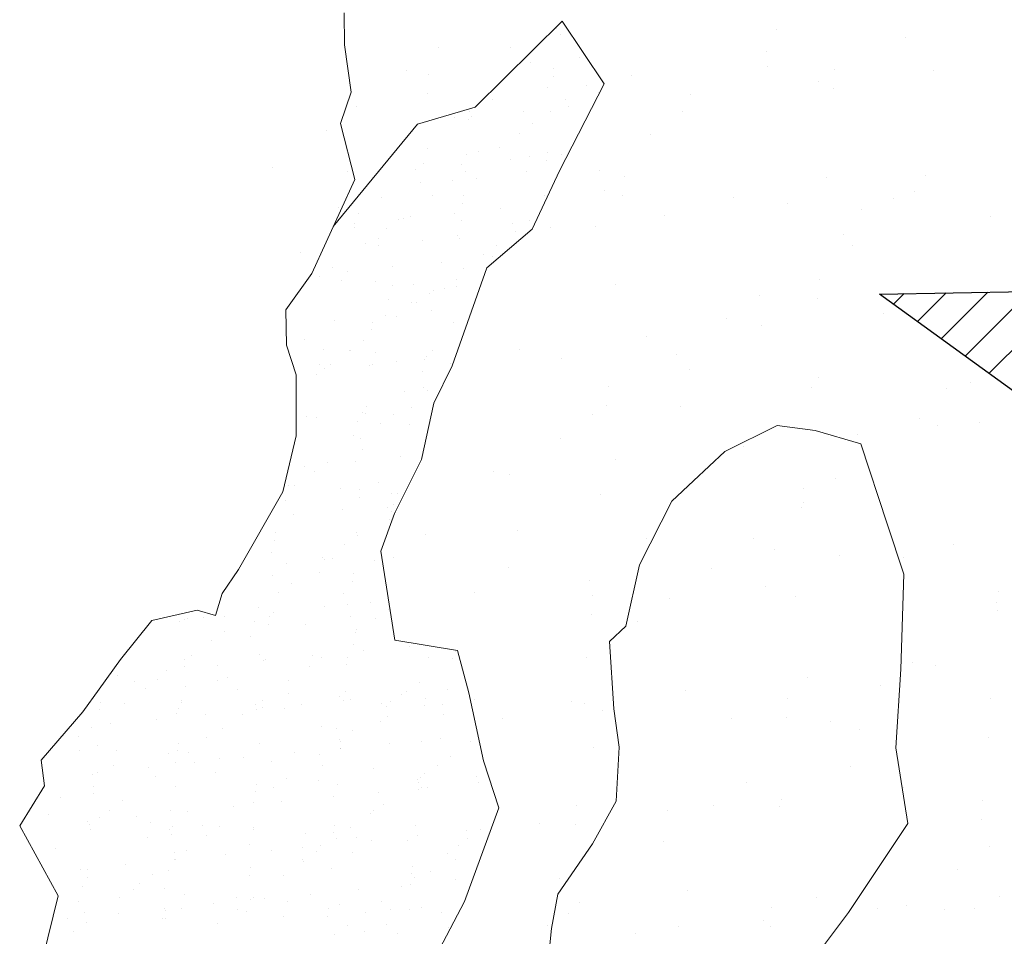
# Model space of a CAD drawing. Units: inches. Extents: x 1986 to 21484, y -1816 to 2016.
# Tile 58 of 85: x 3646.214 to 3651.423, y 1887.486 to 1892.332. Entities that reach past the tile are written whole.
import ezdxf

# ---------------------------------------------------------------- set-up
doc = ezdxf.new("R2010")
doc.units = ezdxf.units.IN
doc.layers.add('L-PLNT', color=84, linetype='Continuous', lineweight=13)
doc.layers.add('vfolha2', color=110, linetype='Continuous')

# ---------------------------------------------------------------- blocks, each defined once
blk = doc.blocks.new('arbusto_PB_verde_grande')
at = {"layer": 'vfolha2'}
h = blk.add_hatch(dxfattribs=at)
h.set_pattern_fill('ANSI31', color=256, scale=0.05, style=0)
h.set_pattern_definition([(45, (-2446.5133113, 50.986076), (-0.004419417382, 0.004419417382), [])])
h.paths.add_polyline_path([(0.02944, 0.35651), (0.00028, 0.09048), (0.02625, -0.03934), (0.047, 0.06233), (0.06189, 0.09731), (0.09372, 0.26573), (0.09955, 0.43473), (0.08789, 0.61313), (0.0645, 0.72266), (0.04988, 0.6851), (0.0236, 0.51294)])
h.paths.add_polyline_path([(0.30106, 0.43789), (0.14225, 0.24871), (0.26685, 0.30022)])
h.paths.add_polyline_path([(0.37995, 0.22817), (0.23697, 0.15193), (0.18428, 0.09364), (0.11122, 0.04358), (0.02625, -0.03934), (0.28061, 0.04667), (0.36829, 0.07798), (0.46756, 0.11239), (0.61068, 0.19376), (0.71585, 0.27823), (0.55813, 0.25948)])
h.paths.add_polyline_path([(0.56101, -0.29441), (0.72752, -0.32573), (0.59024, -0.2412), (0.42962, -0.15982), (0.02625, -0.03934), (0.14922, -0.14107), (0.18838, -0.16604), (0.41501, -0.24435)])
h.paths.add_polyline_path([(-0.27429, -0.44776), (-0.30352, -0.72628), (-0.23923, -0.64175), (-0.15457, -0.45716), (0.02625, -0.03934), (-0.16328, -0.25376)])
h.paths.add_polyline_path([(-0.51963, -0.24744), (-0.67736, -0.32573), (-0.59558, -0.35072), (-0.40574, -0.32882), (-0.21007, -0.20995), (0.02625, -0.03934), (-0.14874, -0.06595), (-0.31518, -0.09101), (-0.41452, -0.15048)])
h.paths.add_polyline_path([(-0.52546, 0.25007), (-0.70947, 0.24698), (-0.51963, 0.1093), (-0.32979, 0.02167), (-0.07567, -0.0128), (-0.04234, -0.02148), (-0.35024, 0.1312)])
for p, q in [((-0.70947, 0.24698), (-0.52546, 0.25007)), ((-0.51963, 0.1093), (-0.70947, 0.24698))]:
    blk.add_line(p, q, dxfattribs=at)
blk = doc.blocks.new('PLANT-SHRUB')
for p, q in [((2174.2393, 1875.2002), (2174.2393, 1875.2002)), ((2174.3788, 1875.1543), (2174.3788, 1875.1543)), ((2174.4979, 1875.0482), (2174.4979, 1875.0482)), ((2174.0964, 1874.9681), (2174.0964, 1874.9681)), ((2174.3044, 1874.9407), (2174.3044, 1874.9407)), ((2174.6293, 1874.8979), (2174.6293, 1874.8979)), ((2174.0311, 1874.8357), (2174.0311, 1874.8357)), ((2174.7545, 1874.8049), (2174.7545, 1874.8049)), ((2173.9574, 1874.7682), (2173.9574, 1874.7682)), ((2175.1665, 1874.7618), (2174.8807, 1874.7126)), ((2174.8807, 1874.7126), (2174.3288, 1874.5846)), ((2174.3288, 1874.5846), (2174.1022, 1874.2498)), ((2173.7058, 1874.5436), (2173.7058, 1874.5436)), ((2174.9504, 1874.5413), (2174.9504, 1874.5413)), ((2175.2326, 1874.4849), (2175.2326, 1874.4849)), ((2174.2141, 1874.4301), (2174.2141, 1874.4301)), ((2175.2365, 1874.4351), (2175.2365, 1874.4351)), ((2173.5596, 1874.4037), (2173.5596, 1874.4037)), ((2175.1589, 1874.4174), (2175.1589, 1874.4174)), ((2174.1022, 1874.2498), (2173.7967, 1873.9642)), ((2174.1022, 1874.2498), (2174.1022, 1874.2498)), ((2174.3436, 1874.1548), (2174.3436, 1874.1548)), ((2175.5883, 1874.1525), (2175.5883, 1874.1525)), ((2173.2119, 1874.085), (2173.2119, 1874.085)), ((2173.6499, 1874.0737), (2173.6499, 1874.0737)), ((2173.1383, 1874.0175), (2173.1383, 1874.0175)), ((2173.185, 1874.0533), (2173.185, 1874.0533)), ((2174.1751, 1874.0474), (2174.1751, 1874.0474)), ((2174.7293, 1874.0348), (2174.7293, 1874.0348)), ((2174.7611, 1874.0529), (2174.7611, 1874.0529)), ((2175.4197, 1874.0451), (2175.4197, 1874.0451)), ((2175.7755, 1874.0214), (2175.7755, 1874.0214)), ((2176.0829, 1873.6984), (2176.4771, 1874.043)), ((2173.7967, 1873.9642), (2173.4419, 1873.6097)), ((2173.7279, 1873.9818), (2173.7279, 1873.9818)), ((2173.9359, 1873.9544), (2173.9359, 1873.9544)), ((2174.2608, 1873.9116), (2174.2608, 1873.9116)), ((2174.8037, 1873.8402), (2174.8037, 1873.8402)), ((2175.0117, 1873.8128), (2175.0117, 1873.8128)), ((2175.3367, 1873.77), (2175.3367, 1873.77)), ((2174.4134, 1873.7343), (2174.4134, 1873.7343)), ((2175.8795, 1873.6985), (2175.8795, 1873.6985)), ((2175.9351, 1873.5901), (2176.0829, 1873.6984)), ((2175.9626, 1873.7021), (2175.9626, 1873.7021)), ((2173.1427, 1873.6734), (2173.1427, 1873.6734)), ((2174.1889, 1873.6601), (2174.1889, 1873.6601)), ((2174.3397, 1873.6667), (2174.3397, 1873.6667)), ((2175.2113, 1873.665), (2175.2113, 1873.665)), ((2176.0876, 1873.6711), (2176.0876, 1873.6711)), ((2173.4419, 1873.6097), (2173.3237, 1873.3537)), ((2175.6198, 1873.5211), (2175.9351, 1873.5901)), ((2173.383, 1873.5428), (2173.383, 1873.5428)), ((2174.6276, 1873.5405), (2174.6276, 1873.5405)), ((2175.8722, 1873.5382), (2175.8722, 1873.5382)), ((2175.3734, 1873.4424), (2175.6198, 1873.5211)), ((2175.1665, 1873.2454), (2175.3734, 1873.4424)), ((2175.6149, 1873.3835), (2175.6149, 1873.3835)), ((2173.3237, 1873.3537), (2173.1364, 1872.95)), ((2176.5897, 1873.3742), (2176.3217, 1873.2797)), ((2172.6023, 1873.2987), (2172.6023, 1873.2987)), ((2173.6247, 1873.3036), (2173.6247, 1873.3036)), ((2173.9419, 1873.3022), (2173.9419, 1873.3022)), ((2175.5412, 1873.316), (2175.5412, 1873.316)), ((2176.3217, 1873.2797), (2175.8488, 1873.0435)), ((2176.4785, 1873.3241), (2176.4785, 1873.3241)), ((2174.7042, 1873.2647), (2174.7042, 1873.2647)), ((2175.0482, 1873.078), (2175.1665, 1873.2454)), ((2175.1665, 1873.2454), (2175.1665, 1873.2454)), ((2175.7503, 1873.2513), (2175.7503, 1873.2513)), ((2176.4488, 1873.2405), (2176.4488, 1873.2405)), ((2172.2836, 1873.1371), (2172.2836, 1873.1371)), ((2172.7762, 1873.1562), (2172.7762, 1873.1562)), ((2174.0209, 1873.154), (2174.0209, 1873.154)), ((2175.2655, 1873.1517), (2175.2655, 1873.1517)), ((2176.2757, 1873.164), (2176.2757, 1873.164)), ((2176.5101, 1873.1494), (2176.5101, 1873.1494)), ((2176.6941, 1873.1587), (2176.6941, 1873.1587)), ((2172.4916, 1873.1097), (2172.4916, 1873.1097)), ((2174.8216, 1872.8023), (2175.0482, 1873.078)), ((2176.2061, 1873.0859), (2176.2061, 1873.0859)), ((2176.5617, 1873.1098), (2176.5617, 1873.1098)), ((2176.704, 1873.085), (2176.704, 1873.085)), ((2172.6077, 1873.0489), (2172.6077, 1873.0489)), ((2172.8165, 1873.067), (2172.8165, 1873.067)), ((2173.8523, 1873.0466), (2173.8523, 1873.0466)), ((2175.097, 1873.0443), (2175.097, 1873.0443)), ((2175.8488, 1873.0435), (2175.7385, 1872.8072)), ((2175.9984, 1873.062), (2175.9984, 1873.062)), ((2176.0816, 1873.051), (2176.0816, 1873.051)), ((2176.1387, 1873.043), (2176.1387, 1873.043)), ((2176.2116, 1873.0339), (2176.2116, 1873.0339)), ((2176.3416, 1873.0421), (2176.3416, 1873.0421)), ((2176.6365, 1873.0421), (2176.6365, 1873.0421)), ((2176.8163, 1873.0327), (2176.8163, 1873.0327)), ((2173.3594, 1872.9955), (2173.3594, 1872.9955)), ((2173.5674, 1872.9681), (2173.5674, 1872.9681)), ((2173.5942, 1872.9836), (2173.5942, 1872.9836)), ((2176.0595, 1873.0141), (2176.0595, 1873.0141)), ((2176.4227, 1872.9824), (2176.4227, 1872.9824)), ((2176.4288, 1873.0053), (2176.4288, 1873.0053)), ((2176.4685, 1873.0161), (2176.4685, 1873.0161)), ((2176.512, 1872.9944), (2176.512, 1872.9944)), ((2176.6419, 1872.9773), (2176.6419, 1872.9773)), ((2176.7427, 1872.9652), (2176.7427, 1872.9652)), ((2173.1364, 1872.95), (2173.2646, 1872.7334)), ((2173.5205, 1872.9161), (2173.5205, 1872.9161)), ((2173.8924, 1872.9253), (2173.8924, 1872.9253)), ((2175.1434, 1872.9514), (2175.1434, 1872.9514)), ((2176.3932, 1872.9554), (2176.3932, 1872.9554)), ((2176.8591, 1872.9487), (2176.8591, 1872.9487)), ((2176.9423, 1872.9377), (2176.9423, 1872.9377)), ((2173.1176, 1872.9033), (2173.1176, 1872.9033)), ((2174.1637, 1872.89), (2174.1637, 1872.89)), ((2175.1861, 1872.8949), (2175.1861, 1872.8949)), ((2175.8338, 1872.8715), (2175.8338, 1872.8715)), ((2174.4352, 1872.8539), (2174.4352, 1872.8539)), ((2174.6433, 1872.8265), (2174.6433, 1872.8265)), ((2175.8218, 1872.8411), (2175.8218, 1872.8411)), ((2176.2341, 1872.8096), (2176.2341, 1872.8096)), ((2176.2656, 1872.856), (2176.2656, 1872.856)), ((2176.2656, 1872.856), (2176.2656, 1872.856)), ((2176.3197, 1872.8402), (2176.3197, 1872.8402)), ((2176.6841, 1872.8506), (2176.6841, 1872.8506)), ((2176.8175, 1872.8393), (2176.8175, 1872.8393)), ((2176.8738, 1872.8151), (2176.8738, 1872.8151)), ((2176.9032, 1872.8421), (2176.9032, 1872.8421)), ((2174.4274, 1872.6152), (2174.7033, 1872.8023)), ((2174.7033, 1872.8023), (2174.8216, 1872.8023)), ((2174.9682, 1872.7837), (2174.9682, 1872.7837)), ((2175.7385, 1872.8072), (2175.5494, 1872.4923)), ((2173.2646, 1872.7334), (2173.3927, 1872.5758)), ((2175.511, 1872.7122), (2175.511, 1872.7122)), ((2176.0494, 1872.7061), (2176.0494, 1872.7061)), ((2176.4584, 1872.708), (2176.4584, 1872.708)), ((2175.7191, 1872.6848), (2175.7191, 1872.6848)), ((2175.851, 1872.6675), (2175.851, 1872.6675)), ((2175.9342, 1872.6565), (2175.9342, 1872.6565)), ((2176.0655, 1872.6551), (2176.0655, 1872.6551)), ((2176.077, 1872.6856), (2176.077, 1872.6856)), ((2176.095, 1872.6821), (2176.095, 1872.6821)), ((2176.5748, 1872.6847), (2176.5748, 1872.6847)), ((2176.7147, 1872.6693), (2176.7147, 1872.6693)), ((2176.8902, 1872.6925), (2176.8902, 1872.6925)), ((2177.0727, 1872.6838), (2177.0727, 1872.6838)), ((2174.0726, 1872.4872), (2174.4274, 1872.6152)), ((2174.7957, 1872.6328), (2174.7957, 1872.6328)), ((2176.0096, 1872.6426), (2176.0096, 1872.6426)), ((2176.044, 1872.6421), (2176.044, 1872.6421)), ((2176.0642, 1872.6394), (2176.0642, 1872.6394)), ((2176.2814, 1872.6108), (2176.2814, 1872.6108)), ((2176.3448, 1872.6007), (2176.3448, 1872.6007)), ((2176.5074, 1872.6417), (2176.5074, 1872.6417)), ((2177.0053, 1872.6408), (2177.0053, 1872.6408)), ((2173.1227, 1872.5516), (2173.1227, 1872.5516)), ((2173.3927, 1872.5758), (2173.6883, 1872.4872)), ((2174.722, 1872.5653), (2174.722, 1872.5653)), ((2175.8237, 1872.5635), (2175.8237, 1872.5635)), ((2176.3646, 1872.5999), (2176.3646, 1872.5999)), ((2176.4945, 1872.5827), (2176.4945, 1872.5827)), ((2176.5869, 1872.5706), (2176.5869, 1872.5706)), ((2176.7117, 1872.5542), (2176.7117, 1872.5542)), ((2171.8156, 1872.5442), (2171.8156, 1872.5442)), ((2172.5771, 1872.5286), (2172.5771, 1872.5286)), ((2173.0602, 1872.5419), (2173.0602, 1872.5419)), ((2173.5995, 1872.5335), (2173.5995, 1872.5335)), ((2174.3048, 1872.5397), (2174.3048, 1872.5397)), ((2175.5495, 1872.5374), (2175.5495, 1872.5374)), ((2175.9064, 1872.5093), (2175.9064, 1872.5093)), ((2176.2555, 1872.5479), (2176.2555, 1872.5479)), ((2176.5461, 1872.5148), (2176.5461, 1872.5148)), ((2176.5756, 1872.5418), (2176.5756, 1872.5418)), ((2176.674, 1872.5426), (2176.674, 1872.5426)), ((2176.7941, 1872.5352), (2176.7941, 1872.5352)), ((2176.7949, 1872.5432), (2176.7949, 1872.5432)), ((2176.7949, 1872.5432), (2176.7949, 1872.5432)), ((2176.9249, 1872.5261), (2176.9249, 1872.5261)), ((2177.083, 1872.5446), (2177.083, 1872.5446)), ((2177.1198, 1872.5004), (2177.1198, 1872.5004)), ((2177.142, 1872.4975), (2177.142, 1872.4975)), ((2177.1952, 1872.5289), (2177.1952, 1872.5289)), ((2173.6883, 1872.4872), (2173.9149, 1872.4872)), ((2173.9149, 1872.4872), (2174.0726, 1872.4872)), ((2174.679, 1872.4946), (2174.679, 1872.4946)), ((2175.5494, 1872.4923), (2175.439, 1872.2875)), ((2175.7252, 1872.4812), (2175.7252, 1872.4812)), ((2176.7476, 1872.4861), (2176.7476, 1872.4861)), ((2177.2252, 1872.4865), (2177.2252, 1872.4865)), ((2177.3552, 1872.4694), (2177.3552, 1872.4694)), ((2175.6209, 1872.4034), (2175.6209, 1872.4034)), ((2175.6927, 1872.4408), (2175.6927, 1872.4408)), ((2176.0394, 1872.398), (2176.0394, 1872.398)), ((2176.1906, 1872.4399), (2176.1906, 1872.4399)), ((2176.4483, 1872.4), (2176.4483, 1872.4)), ((2176.6884, 1872.439), (2176.6884, 1872.439)), ((2177.0562, 1872.4015), (2177.0562, 1872.4015)), ((2177.1863, 1872.4381), (2177.1863, 1872.4381)), ((2175.7378, 1872.3549), (2175.7378, 1872.3549)), ((2175.7673, 1872.3819), (2175.7673, 1872.3819)), ((2176.387, 1872.369), (2176.387, 1872.369)), ((2176.8801, 1872.3844), (2176.8801, 1872.3844)), ((2177.0267, 1872.3745), (2177.0267, 1872.3745)), ((2177.2986, 1872.3791), (2177.2986, 1872.3791)), ((2175.4865, 1872.3015), (2175.4865, 1872.3015)), ((2175.439, 1872.2875), (2175.6439, 1872.0198)), ((2175.45, 1872.2862), (2175.45, 1872.2862)), ((2175.7036, 1872.2729), (2175.7036, 1872.2729)), ((2175.7868, 1872.262), (2175.7868, 1872.262)), ((2175.8137, 1872.2554), (2175.8137, 1872.2554)), ((2175.8805, 1872.2423), (2175.8805, 1872.2423)), ((2175.9168, 1872.2449), (2175.9168, 1872.2449)), ((2175.9479, 1872.2853), (2175.9479, 1872.2853)), ((2175.9971, 1872.2821), (2175.9971, 1872.2821)), ((2176.2455, 1872.2399), (2176.2455, 1872.2399)), ((2176.2479, 1872.2416), (2176.2479, 1872.2416)), ((2176.3783, 1872.2414), (2176.3783, 1872.2414)), ((2176.4457, 1872.2844), (2176.4457, 1872.2844)), ((2176.8762, 1872.2405), (2176.8762, 1872.2405)), ((2176.9436, 1872.2835), (2176.9436, 1872.2835)), ((2177.0729, 1872.2365), (2177.0729, 1872.2365)), ((2177.374, 1872.2396), (2177.374, 1872.2396)), ((2177.4414, 1872.2826), (2177.4414, 1872.2826)), ((2177.5367, 1872.2612), (2177.5367, 1872.2612)), ((2177.5463, 1872.2499), (2177.5463, 1872.2499)), ((2172.775, 1872.233), (2172.775, 1872.233)), ((2174.3242, 1872.2008), (2174.3242, 1872.2008)), ((2175.5787, 1872.2091), (2175.5787, 1872.2091)), ((2175.9235, 1872.2145), (2175.9235, 1872.2145)), ((2176.134, 1872.2163), (2176.134, 1872.2163)), ((2176.2172, 1872.2053), (2176.2172, 1872.2053)), ((2176.2184, 1872.2145), (2176.2184, 1872.2145)), ((2176.3471, 1872.1882), (2176.3471, 1872.1882)), ((2176.6639, 1872.2346), (2176.6639, 1872.2346)), ((2176.8676, 1872.2287), (2176.8676, 1872.2287)), ((2177.5047, 1872.221), (2177.5047, 1872.221)), ((2177.5073, 1872.2342), (2177.5073, 1872.2342)), ((2171.9151, 1872.1508), (2171.9151, 1872.1508)), ((2172.0129, 1872.1721), (2172.0129, 1872.1721)), ((2172.4534, 1872.1554), (2172.4534, 1872.1554)), ((2172.7014, 1872.1655), (2172.7014, 1872.1655)), ((2173.0924, 1872.1332), (2173.0924, 1872.1332)), ((2173.6981, 1872.1531), (2173.6981, 1872.1531)), ((2174.9427, 1872.1509), (2174.9427, 1872.1509)), ((2176.1873, 1872.1486), (2176.1873, 1872.1486)), ((2176.5643, 1872.1596), (2176.5643, 1872.1596)), ((2176.6475, 1872.1487), (2176.6475, 1872.1487)), ((2177.432, 1872.1464), (2177.432, 1872.1464)), ((2172.1231, 1872.1234), (2172.1231, 1872.1234)), ((2172.448, 1872.0807), (2172.448, 1872.0807)), ((2174.1386, 1872.1199), (2174.1386, 1872.1199)), ((2175.161, 1872.1248), (2175.161, 1872.1248)), ((2175.6108, 1872.0953), (2175.6108, 1872.0953)), ((2176.0293, 1872.09), (2176.0293, 1872.09)), ((2176.2404, 1872.0859), (2176.2404, 1872.0859)), ((2176.4382, 1872.092), (2176.4382, 1872.092)), ((2176.7285, 1872.1012), (2176.7285, 1872.1012)), ((2176.7775, 1872.1316), (2176.7775, 1872.1316)), ((2176.9946, 1872.103), (2176.9946, 1872.103)), ((2177.0778, 1872.092), (2177.0778, 1872.092)), ((2177.3482, 1872.0884), (2177.3482, 1872.0884)), ((2172.2849, 1872.048), (2172.2849, 1872.048)), ((2173.5295, 1872.0458), (2173.5295, 1872.0458)), ((2174.7742, 1872.0435), (2174.7742, 1872.0435)), ((2176.0188, 1872.0413), (2176.0188, 1872.0413)), ((2176.0593, 1872.0687), (2176.0593, 1872.0687)), ((2176.0615, 1872.0396), (2176.0615, 1872.0396)), ((2176.5593, 1872.0387), (2176.5593, 1872.0387)), ((2176.699, 1872.0742), (2176.699, 1872.0742)), ((2176.87, 1872.0764), (2176.87, 1872.0764)), ((2177.0572, 1872.0377), (2177.0572, 1872.0377)), ((2177.2078, 1872.0749), (2177.2078, 1872.0749)), ((2177.2634, 1872.039), (2177.2634, 1872.039)), ((2177.2866, 1872.0725), (2177.2866, 1872.0725)), ((2177.2885, 1872.0711), (2177.2885, 1872.0711)), ((2177.4249, 1872.0463), (2177.4249, 1872.0463)), ((2177.5082, 1872.0354), (2177.5082, 1872.0354)), ((2177.555, 1872.0368), (2177.555, 1872.0368)), ((2177.6975, 1872.073), (2177.6975, 1872.073)), ((2172.9909, 1872.0092), (2172.9909, 1872.0092)), ((2173.1989, 1871.9818), (2173.1989, 1871.9818)), ((2175.6439, 1872.0198), (2175.376, 1871.626)), ((2177.6381, 1872.0183), (2177.6381, 1872.0183)), ((2177.8553, 1871.9897), (2177.8553, 1871.9897)), ((2178.1671, 1871.9818), (2177.8688, 1871.7874)), ((2177.9385, 1871.9787), (2177.9385, 1871.9787)), ((2173.5239, 1871.939), (2173.5239, 1871.939)), ((2175.8036, 1871.9474), (2175.8036, 1871.9474)), ((2175.9202, 1871.9413), (2175.9202, 1871.9413)), ((2176.2354, 1871.9319), (2176.2354, 1871.9319)), ((2176.5399, 1871.9284), (2176.5399, 1871.9284)), ((2176.6539, 1871.9265), (2176.6539, 1871.9265)), ((2177.0628, 1871.9285), (2177.0628, 1871.9285)), ((2177.1796, 1871.9339), (2177.1796, 1871.9339)), ((2177.1986, 1871.9313), (2177.1986, 1871.9313)), ((2177.2091, 1871.9609), (2177.2091, 1871.9609)), ((2177.8287, 1871.9481), (2177.8287, 1871.9481)), ((2173.9765, 1871.8822), (2173.9765, 1871.8822)), ((2175.5562, 1871.8784), (2175.5562, 1871.8784)), ((2175.8188, 1871.8849), (2175.8188, 1871.8849)), ((2175.8908, 1871.9143), (2175.8908, 1871.9143)), ((2176.3166, 1871.884), (2176.3166, 1871.884)), ((2176.8145, 1871.8831), (2176.8145, 1871.8831)), ((2177.3123, 1871.8822), (2177.3123, 1871.8822)), ((2177.4946, 1871.9129), (2177.4946, 1871.9129)), ((2177.8102, 1871.8813), (2177.8102, 1871.8813)), ((2177.9131, 1871.9076), (2177.9131, 1871.9076)), ((2174.0667, 1871.8676), (2174.0667, 1871.8676)), ((2174.2748, 1871.8402), (2174.2748, 1871.8402)), ((2175.5257, 1871.85), (2175.5257, 1871.85)), ((2175.6394, 1871.8675), (2175.6394, 1871.8675)), ((2175.7514, 1871.842), (2175.7514, 1871.842)), ((2175.7694, 1871.8504), (2175.7694, 1871.8504)), ((2175.9866, 1871.8218), (2175.9866, 1871.8218)), ((2176.2492, 1871.8411), (2176.2492, 1871.8411)), ((2176.7471, 1871.8402), (2176.7471, 1871.8402)), ((2177.1249, 1871.8638), (2177.1249, 1871.8638)), ((2177.2449, 1871.8393), (2177.2449, 1871.8393)), ((2177.6897, 1871.8206), (2177.6897, 1871.8206)), ((2177.7428, 1871.8384), (2177.7428, 1871.8384)), ((2171.5058, 1871.7718), (2171.5058, 1871.7718)), ((2172.3036, 1871.801), (2172.3036, 1871.801)), ((2173.9028, 1871.8147), (2173.9028, 1871.8147)), ((2174.5997, 1871.7974), (2174.5997, 1871.7974)), ((2175.6007, 1871.7873), (2175.6007, 1871.7873)), ((2175.7316, 1871.7685), (2175.7316, 1871.7685)), ((2176.0192, 1871.782), (2176.0192, 1871.782)), ((2176.0698, 1871.8108), (2176.0698, 1871.8108)), ((2176.1997, 1871.7937), (2176.1997, 1871.7937)), ((2176.3713, 1871.774), (2176.3713, 1871.774)), ((2176.4008, 1871.801), (2176.4008, 1871.801)), ((2176.4282, 1871.7839), (2176.4282, 1871.7839)), ((2176.86, 1871.7684), (2176.86, 1871.7684)), ((2177.0205, 1871.7881), (2177.0205, 1871.7881)), ((2177.6602, 1871.7936), (2177.6602, 1871.7936)), ((2177.8688, 1871.7874), (2177.7634, 1871.3785)), ((2172.552, 1871.7585), (2172.552, 1871.7585)), ((2173.5743, 1871.7634), (2173.5743, 1871.7634)), ((2174.6538, 1871.7245), (2174.6538, 1871.7245)), ((2175.1425, 1871.7259), (2175.1425, 1871.7259)), ((2176.4169, 1871.7651), (2176.4169, 1871.7651)), ((2176.5001, 1871.7542), (2176.5001, 1871.7542)), ((2176.6301, 1871.7371), (2176.6301, 1871.7371)), ((2176.7224, 1871.7161), (2176.7224, 1871.7161)), ((2177.2784, 1871.763), (2177.2784, 1871.763)), ((2177.6874, 1871.765), (2177.6874, 1871.765)), ((2175.3506, 1871.6985), (2175.3506, 1871.6985)), ((2175.7, 1871.7111), (2175.7, 1871.7111)), ((2176.8472, 1871.7085), (2176.8472, 1871.7085)), ((2176.9304, 1871.6975), (2176.9304, 1871.6975)), ((2177.0604, 1871.6804), (2177.0604, 1871.6804)), ((2175.376, 1871.626), (2175.1869, 1871.5315)), ((2175.3846, 1871.6374), (2175.3846, 1871.6374)), ((2175.4345, 1871.6401), (2175.4345, 1871.6401)), ((2175.5631, 1871.614), (2175.5631, 1871.614)), ((2175.5926, 1871.641), (2175.5926, 1871.641)), ((2175.6755, 1871.6558), (2175.6755, 1871.6558)), ((2175.7935, 1871.6394), (2175.7935, 1871.6394)), ((2175.9323, 1871.6392), (2175.9323, 1871.6392)), ((2176.2122, 1871.6282), (2176.2122, 1871.6282)), ((2176.2253, 1871.6238), (2176.2253, 1871.6238)), ((2176.4302, 1871.6383), (2176.4302, 1871.6383)), ((2176.6438, 1871.6185), (2176.6438, 1871.6185)), ((2176.8519, 1871.6337), (2176.8519, 1871.6337)), ((2176.8814, 1871.6607), (2176.8814, 1871.6607)), ((2176.9281, 1871.6374), (2176.9281, 1871.6374)), ((2177.0527, 1871.6204), (2177.0527, 1871.6204)), ((2177.2775, 1871.6518), (2177.2775, 1871.6518)), ((2177.3608, 1871.6409), (2177.3608, 1871.6409)), ((2177.4259, 1871.6365), (2177.4259, 1871.6365)), ((2177.4907, 1871.6237), (2177.4907, 1871.6237)), ((2177.5011, 1871.6478), (2177.5011, 1871.6478)), ((2176.2184, 1871.5843), (2176.2184, 1871.5843)), ((2177.4845, 1871.6049), (2177.4845, 1871.6049)), ((2177.7079, 1871.5952), (2177.7079, 1871.5952)), ((2171.4928, 1871.5434), (2171.4928, 1871.5434)), ((2172.7374, 1871.5411), (2172.7374, 1871.5411)), ((2173.982, 1871.5389), (2173.982, 1871.5389)), ((2175.1869, 1871.5315), (2174.8874, 1871.4213)), ((2175.178, 1871.5314), (2175.178, 1871.5314)), ((2175.1869, 1871.5315), (2175.1869, 1871.5315)), ((2175.1917, 1871.5125), (2175.1917, 1871.5125)), ((2175.2267, 1871.5366), (2175.2267, 1871.5366)), ((2176.4264, 1871.5569), (2176.4264, 1871.5569)), ((2176.4713, 1871.5343), (2176.4713, 1871.5343)), ((2176.7513, 1871.5141), (2176.7513, 1871.5141)), ((2177.362, 1871.5204), (2177.362, 1871.5204)), ((2171.9559, 1871.4823), (2171.9559, 1871.4823)), ((2175.1043, 1871.4639), (2175.1043, 1871.4639)), ((2175.1589, 1871.4948), (2175.1589, 1871.4948)), ((2175.1918, 1871.4855), (2175.1918, 1871.4855)), ((2175.404, 1871.4682), (2175.404, 1871.4682)), ((2175.4088, 1871.4839), (2175.4088, 1871.4839)), ((2175.492, 1871.473), (2175.492, 1871.473)), ((2175.5907, 1871.4793), (2175.5907, 1871.4793)), ((2175.622, 1871.4558), (2175.622, 1871.4558)), ((2175.6897, 1871.4846), (2175.6897, 1871.4846)), ((2176.0091, 1871.4739), (2176.0091, 1871.4739)), ((2176.0437, 1871.4737), (2176.0437, 1871.4737)), ((2176.0731, 1871.5007), (2176.0731, 1871.5007)), ((2176.1875, 1871.4837), (2176.1875, 1871.4837)), ((2176.4181, 1871.4759), (2176.4181, 1871.4759)), ((2176.6854, 1871.4828), (2176.6854, 1871.4828)), ((2176.6928, 1871.4879), (2176.6928, 1871.4879)), ((2176.7271, 1871.4992), (2176.7271, 1871.4992)), ((2176.8499, 1871.4603), (2176.8499, 1871.4603)), ((2177.1832, 1871.4819), (2177.1832, 1871.4819)), ((2177.2684, 1871.455), (2177.2684, 1871.455)), ((2177.3325, 1871.4934), (2177.3325, 1871.4934)), ((2171.8822, 1871.4148), (2171.8822, 1871.4148)), ((2173.505, 1871.4502), (2173.505, 1871.4502)), ((2174.8874, 1871.4213), (2174.6352, 1871.248)), ((2174.8874, 1871.4213), (2174.8874, 1871.4213)), ((2175.1244, 1871.4426), (2175.1244, 1871.4426)), ((2175.6222, 1871.4417), (2175.6222, 1871.4417)), ((2175.8392, 1871.4273), (2175.8392, 1871.4273)), ((2175.9224, 1871.4163), (2175.9224, 1871.4163)), ((2176.1201, 1871.4408), (2176.1201, 1871.4408)), ((2176.6179, 1871.4399), (2176.6179, 1871.4399)), ((2177.1158, 1871.439), (2177.1158, 1871.439)), ((2177.2942, 1871.4427), (2177.2942, 1871.4427)), ((2177.5022, 1871.4153), (2177.5022, 1871.4153)), ((2177.6136, 1871.438), (2177.6136, 1871.438)), ((2171.9877, 1871.402), (2171.9877, 1871.402)), ((2173.0672, 1871.3631), (2173.0672, 1871.3631)), ((2175.1358, 1871.3547), (2175.1358, 1871.3547)), ((2176.0523, 1871.3992), (2176.0523, 1871.3992)), ((2176.2695, 1871.3706), (2176.2695, 1871.3706)), ((2176.3527, 1871.3596), (2176.3527, 1871.3596)), ((2176.5537, 1871.3604), (2176.5537, 1871.3604)), ((2177.7634, 1871.3785), (2177.5228, 1871.3129)), ((2174.1134, 1871.3498), (2174.1134, 1871.3498)), ((2174.956, 1871.3347), (2174.956, 1871.3347)), ((2175.2354, 1871.3138), (2175.2354, 1871.3138)), ((2175.2649, 1871.3408), (2175.2649, 1871.3408)), ((2175.3745, 1871.3294), (2175.3745, 1871.3294)), ((2175.7835, 1871.3313), (2175.7835, 1871.3313)), ((2175.8846, 1871.3279), (2175.8846, 1871.3279)), ((2176.2152, 1871.3158), (2176.2152, 1871.3158)), ((2176.2152, 1871.3158), (2176.2152, 1871.3158)), ((2176.4827, 1871.3425), (2176.4827, 1871.3425)), ((2176.5243, 1871.3334), (2176.5243, 1871.3334)), ((2176.6337, 1871.3104), (2176.6337, 1871.3104)), ((2176.6998, 1871.3139), (2176.6998, 1871.3139)), ((2176.783, 1871.303), (2176.783, 1871.303)), ((2177.0427, 1871.3124), (2177.0427, 1871.3124)), ((2177.1734, 1871.3475), (2177.1734, 1871.3475)), ((2177.2614, 1871.3024), (2177.2614, 1871.3024)), ((2177.5228, 1871.3129), (2177.4426, 1871.2036)), ((2174.6352, 1871.248), (2174.4303, 1871.1693)), ((2176.247, 1871.2765), (2176.1409, 1871.2146)), ((2176.298, 1871.1891), (2176.247, 1871.2765)), ((2176.913, 1871.2859), (2176.913, 1871.2859)), ((2177.1302, 1871.2573), (2177.1302, 1871.2573)), ((2177.2134, 1871.2463), (2177.2134, 1871.2463)), ((2174.8075, 1871.2407), (2174.8075, 1871.2407)), ((2175.3054, 1871.2398), (2175.3054, 1871.2398)), ((2175.7455, 1871.2005), (2175.7455, 1871.2005)), ((2175.8032, 1871.2389), (2175.8032, 1871.2389)), ((2176.1409, 1871.2146), (2175.9918, 1871.1818)), ((2176.3011, 1871.238), (2176.3011, 1871.238)), ((2176.7989, 1871.2371), (2176.7989, 1871.2371)), ((2177.0343, 1871.2201), (2177.0343, 1871.2201)), ((2177.4426, 1871.2036), (2177.1073, 1871.1672)), ((2172.1307, 1871.1546), (2172.1307, 1871.1546)), ((2173.3753, 1871.1523), (2173.3753, 1871.1523)), ((2174.4303, 1871.1693), (2173.9417, 1870.9173)), ((2174.4272, 1871.1538), (2174.4272, 1871.1538)), ((2174.4303, 1871.1693), (2174.4303, 1871.1693)), ((2174.614, 1871.1746), (2174.614, 1871.1746)), ((2174.6199, 1871.1501), (2174.6199, 1871.1501)), ((2174.7399, 1871.1848), (2174.7399, 1871.1848)), ((2174.8311, 1871.146), (2174.8311, 1871.146)), ((2175.0763, 1871.168), (2175.0763, 1871.168)), ((2175.1488, 1871.1868), (2175.1488, 1871.1868)), ((2175.9918, 1871.1818), (2175.5398, 1871.0434)), ((2175.5806, 1871.1712), (2175.5806, 1871.1712)), ((2175.716, 1871.1735), (2175.716, 1871.1735)), ((2176.5094, 1871.0652), (2176.298, 1871.1891)), ((2176.3651, 1871.1876), (2176.3651, 1871.1876)), ((2176.3794, 1871.1806), (2176.3794, 1871.1806)), ((2176.408, 1871.1678), (2176.408, 1871.1678)), ((2176.8398, 1871.1523), (2176.8398, 1871.1523)), ((2177.1073, 1871.1672), (2176.9614, 1871.1381)), ((2177.0048, 1871.1931), (2177.0048, 1871.1931)), ((2172.0795, 1871.0944), (2172.0795, 1871.0944)), ((2173.1573, 1871.1316), (2173.1573, 1871.1316)), ((2174.7065, 1871.0994), (2174.7065, 1871.0994)), ((2174.9143, 1871.1351), (2174.9143, 1871.1351)), ((2175.0443, 1871.118), (2175.0443, 1871.118)), ((2176.7719, 1871.1017), (2176.5094, 1871.0652)), ((2176.9614, 1871.1381), (2176.7719, 1871.1017)), ((2171.9621, 1871.0472), (2171.9621, 1871.0472)), ((2173.0837, 1871.0641), (2173.0837, 1871.0641)), ((2173.2068, 1871.045), (2173.2068, 1871.045)), ((2174.4514, 1871.0427), (2174.4514, 1871.0427)), ((2174.4974, 1871.0431), (2174.4974, 1871.0431)), ((2174.5142, 1871.0422), (2174.5142, 1871.0422)), ((2174.5648, 1871.0861), (2174.5648, 1871.0861)), ((2174.9372, 1871.0405), (2174.9372, 1871.0405)), ((2174.9953, 1871.0422), (2174.9953, 1871.0422)), ((2175.0627, 1871.0852), (2175.0627, 1871.0852)), ((2175.2614, 1871.0894), (2175.2614, 1871.0894)), ((2175.5398, 1871.0434), (2175.2846, 1870.8758)), ((2175.3446, 1871.0784), (2175.3446, 1871.0784)), ((2175.4746, 1871.0613), (2175.4746, 1871.0613)), ((2175.4931, 1871.0413), (2175.4931, 1871.0413)), ((2175.5398, 1871.0434), (2175.5398, 1871.0434)), ((2175.5605, 1871.0843), (2175.5605, 1871.0843)), ((2172.5268, 1870.9884), (2172.5268, 1870.9884)), ((2172.6224, 1871.0229), (2172.6224, 1871.0229)), ((2172.8304, 1870.9955), (2172.8304, 1870.9955)), ((2173.5492, 1870.9933), (2173.5492, 1870.9933)), ((2174.268, 1871.008), (2174.268, 1871.008)), ((2174.9077, 1871.0135), (2174.9077, 1871.0135)), ((2174.946, 1871.0267), (2174.946, 1871.0267)), ((2175.3644, 1871.0213), (2175.3644, 1871.0213)), ((2173.1554, 1870.9527), (2173.1554, 1870.9527)), ((2174.6286, 1870.9544), (2174.6286, 1870.9544)), ((2173.6264, 1870.9331), (2173.3112, 1870.8071)), ((2173.6059, 1870.8934), (2173.6059, 1870.8934)), ((2173.9417, 1870.9173), (2173.6264, 1870.9331)), ((2173.8795, 1870.8977), (2173.8795, 1870.8977)), ((2173.9417, 1870.9173), (2173.9417, 1870.9173)), ((2173.9417, 1870.9173), (2173.9417, 1870.9173)), ((2174.3113, 1870.8821), (2174.3113, 1870.8821)), ((2173.4598, 1870.8481), (2173.4598, 1870.8481)), ((2173.6827, 1870.8422), (2173.6827, 1870.8422)), ((2173.6982, 1870.8813), (2173.6982, 1870.8813)), ((2173.823, 1870.8648), (2173.823, 1870.8648)), ((2173.9063, 1870.8539), (2173.9063, 1870.8539)), ((2173.9063, 1870.8539), (2173.9063, 1870.8539)), ((2174.0362, 1870.8368), (2174.0362, 1870.8368)), ((2174.0995, 1870.8536), (2174.0995, 1870.8536)), ((2174.129, 1870.8806), (2174.129, 1870.8806)), ((2174.1806, 1870.8413), (2174.1806, 1870.8413)), ((2174.6784, 1870.8404), (2174.6784, 1870.8404)), ((2174.7298, 1870.8768), (2174.7298, 1870.8768)), ((2174.7486, 1870.8677), (2174.7486, 1870.8677)), ((2175.2846, 1870.8758), (2175.0644, 1870.6405)), ((2175.1387, 1870.8787), (2175.1387, 1870.8787)), ((2175.1763, 1870.8395), (2175.1763, 1870.8395)), ((2173.3112, 1870.8071), (2172.8226, 1870.6338)), ((2173.3112, 1870.8071), (2173.3112, 1870.8071)), ((2174.2312, 1870.8111), (2174.2312, 1870.8111)), ((2174.2534, 1870.8082), (2174.2534, 1870.8082)), ((2174.3366, 1870.7972), (2174.3366, 1870.7972)), ((2174.3588, 1870.7808), (2174.3588, 1870.7808)), ((2174.4666, 1870.7801), (2174.4666, 1870.7801)), ((2173.2449, 1870.7531), (2173.2449, 1870.7531)), ((2173.6767, 1870.7376), (2173.6767, 1870.7376)), ((2174.0951, 1870.7322), (2174.0951, 1870.7322)), ((2174.5041, 1870.7342), (2174.5041, 1870.7342)), ((2174.6095, 1870.7403), (2174.6095, 1870.7403)), ((2174.6837, 1870.7515), (2174.6837, 1870.7515)), ((2174.7669, 1870.7406), (2174.7669, 1870.7406)), ((2174.7741, 1870.7396), (2174.7741, 1870.7396)), ((2172.6859, 1870.6995), (2172.6859, 1870.6995)), ((2173.2912, 1870.6936), (2173.2912, 1870.6936)), ((2173.3207, 1870.7206), (2173.3207, 1870.7206)), ((2173.44, 1870.6876), (2173.44, 1870.6876)), ((2173.9379, 1870.6867), (2173.9379, 1870.6867)), ((2173.9404, 1870.7078), (2173.9404, 1870.7078)), ((2174.2851, 1870.7133), (2174.2851, 1870.7133)), ((2174.4357, 1870.6858), (2174.4357, 1870.6858)), ((2174.5801, 1870.7133), (2174.5801, 1870.7133)), ((2174.8969, 1870.7235), (2174.8969, 1870.7235)), ((2174.9336, 1870.6849), (2174.9336, 1870.6849)), ((2174.9359, 1870.7186), (2174.9359, 1870.7186)), ((2174.9821, 1870.7122), (2174.9821, 1870.7122)), ((2175.114, 1870.6949), (2175.114, 1870.6949)), ((2172.8226, 1870.6338), (2172.7595, 1870.2401)), ((2172.8226, 1870.6338), (2172.8226, 1870.6338)), ((2172.8747, 1870.6455), (2172.8747, 1870.6455)), ((2173.3726, 1870.6446), (2173.3726, 1870.6446)), ((2173.8704, 1870.6437), (2173.8704, 1870.6437)), ((2174.3683, 1870.6428), (2174.3683, 1870.6428)), ((2174.8662, 1870.6419), (2174.8662, 1870.6419)), ((2175.0644, 1870.6405), (2174.9952, 1870.4908)), ((2172.815, 1870.5836), (2172.815, 1870.5836)), ((2172.8982, 1870.5727), (2172.8982, 1870.5727)), ((2173.042, 1870.593), (2173.042, 1870.593)), ((2173.042, 1870.593), (2173.042, 1870.593)), ((2173.4605, 1870.5877), (2173.4605, 1870.5877)), ((2173.8013, 1870.5803), (2173.8013, 1870.5803)), ((2173.8695, 1870.5896), (2173.8695, 1870.5896)), ((2174.0882, 1870.5797), (2174.0882, 1870.5797)), ((2174.3012, 1870.5741), (2174.3012, 1870.5741)), ((2173.0282, 1870.5556), (2173.0282, 1870.5556)), ((2173.1321, 1870.5478), (2173.1321, 1870.5478)), ((2173.2453, 1870.527), (2173.2453, 1870.527)), ((2173.6592, 1870.538), (2173.6592, 1870.538)), ((2173.7718, 1870.5533), (2173.7718, 1870.5533)), ((2174.421, 1870.5675), (2174.421, 1870.5675)), ((2174.7197, 1870.5687), (2174.7197, 1870.5687)), ((2174.9039, 1870.5358), (2174.9039, 1870.5358)), ((2173.3285, 1870.516), (2173.3285, 1870.516)), ((2173.4585, 1870.4989), (2173.4585, 1870.4989)), ((2173.6756, 1870.4703), (2173.6756, 1870.4703)), ((2174.9952, 1870.4908), (2174.8685, 1870.3527)), ((2172.8259, 1870.4431), (2172.8259, 1870.4431)), ((2172.993, 1870.4204), (2172.993, 1870.4204)), ((2173.0557, 1870.4428), (2173.0557, 1870.4428)), ((2173.2348, 1870.4451), (2173.2348, 1870.4451)), ((2173.5536, 1870.4419), (2173.5536, 1870.4419)), ((2173.6666, 1870.4295), (2173.6666, 1870.4295)), ((2173.7589, 1870.4594), (2173.7589, 1870.4594)), ((2173.8888, 1870.4423), (2173.8888, 1870.4423)), ((2174.0514, 1870.441), (2174.0514, 1870.441)), ((2174.0851, 1870.4242), (2174.0851, 1870.4242)), ((2174.106, 1870.4137), (2174.106, 1870.4137)), ((2174.2524, 1870.413), (2174.2524, 1870.413)), ((2174.2819, 1870.44), (2174.2819, 1870.44)), ((2174.494, 1870.4262), (2174.494, 1870.4262)), ((2174.5493, 1870.4401), (2174.5493, 1870.4401)), ((2172.9636, 1870.3934), (2172.9636, 1870.3934)), ((2173.6127, 1870.4075), (2173.6127, 1870.4075)), ((2174.1892, 1870.4027), (2174.1892, 1870.4027)), ((2174.3192, 1870.3856), (2174.3192, 1870.3856)), ((2173.8873, 1870.3488), (2173.8873, 1870.3488)), ((2174.5363, 1870.357), (2174.5363, 1870.357)), ((2174.6195, 1870.3461), (2174.6195, 1870.3461)), ((2174.8685, 1870.3527), (2174.6381, 1870.3067)), ((2174.7495, 1870.3289), (2174.7495, 1870.3289)), ((2172.813, 1870.2882), (2172.813, 1870.2882)), ((2173.032, 1870.285), (2173.032, 1870.285)), ((2173.3109, 1870.2873), (2173.3109, 1870.2873)), ((2173.4504, 1870.2796), (2173.4504, 1870.2796)), ((2173.4736, 1870.2801), (2173.4736, 1870.2801)), ((2173.8088, 1870.2863), (2173.8088, 1870.2863)), ((2173.8594, 1870.2816), (2173.8594, 1870.2816)), ((2174.0933, 1870.2672), (2174.0933, 1870.2672)), ((2174.6381, 1870.3067), (2174.1312, 1870.0995)), ((2174.2912, 1870.266), (2174.2912, 1870.266)), ((2174.3066, 1870.2854), (2174.3066, 1870.2854)), ((2172.7595, 1870.2401), (2173.4058, 1870.2558)), ((2172.8044, 1870.2476), (2172.8044, 1870.2476)), ((2173.4058, 1870.2558), (2173.6895, 1870.1141)), ((2173.4441, 1870.2531), (2173.4441, 1870.2531)), ((2173.524, 1870.2232), (2173.524, 1870.2232)), ((2173.7413, 1870.2434), (2173.7413, 1870.2434)), ((2174.2392, 1870.2425), (2174.2392, 1870.2425)), ((2173.6895, 1870.1141), (2174.3847, 1870.2031)), ((2174.6035, 1870.1843), (2174.6035, 1870.1843)), ((2173.0525, 1870.1515), (2173.0525, 1870.1515)), ((2173.6895, 1870.1141), (2173.6895, 1870.1141)), ((2174.2971, 1870.1493), (2174.2971, 1870.1493)), ((2174.1312, 1870.0995), (2173.9841, 1869.8328)), ((2173.5396, 1870.0301), (2173.5396, 1870.0301)), ((2174.1286, 1870.0419), (2174.1286, 1870.0419)), ((2173.4659, 1869.9626), (2173.4659, 1869.9626)), ((2173.3297, 1869.895), (2173.3297, 1869.895)), ((2173.5378, 1869.8676), (2173.5378, 1869.8676)), ((2173.9841, 1869.8328), (2173.8287, 1869.75)), ((2173.8627, 1869.8248), (2173.8627, 1869.8248)), ((2174.063, 1869.8096), (2174.063, 1869.8096)), ((2173.8287, 1869.75), (2173.6837, 1869.543)), ((2174.4056, 1869.7533), (2174.4056, 1869.7533)), ((2173.6837, 1869.543), (2173.5698, 1869.4188))]:
    blk.add_line(p, q)

msp = doc.modelspace()

# ---------------------------------------------------------------- block references
at = {"layer": 'L-PLNT', "rotation": 223.1883365522388}
msp.add_blockref('PLANT-SHRUB', (3953.27, 4742.9646), dxfattribs=at)
at = {"layer": 'L-PLNT', "xscale": 24.60366729364114, "yscale": 24.60366729364114, "zscale": 24.60366729364114}
msp.add_blockref('arbusto_PB_verde_grande', (3668.2184, 1884.8051), dxfattribs=at)

doc.saveas('drawing.dxf')
